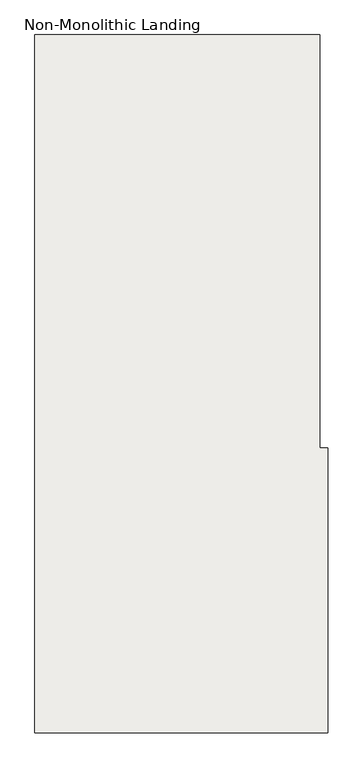
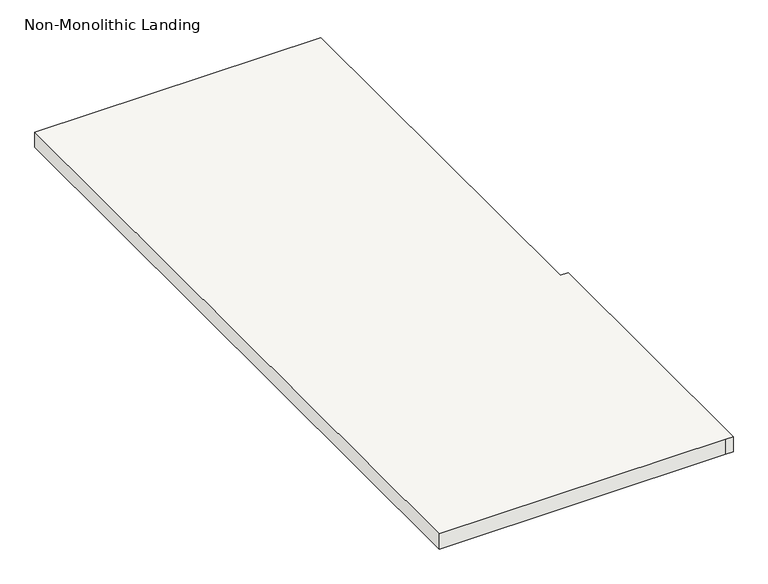
"""IFC4 building model written with IfcOpenShell, lengths in millimetres: slab geometry, Non-Monolithic Landing."""

from ifc_helpers import new_model, si_unit, origin, place, context, project, spatial, faceted_brep, source, transform, mapped, element, save


def non_monolithic_landing_62f4187a(model_context):
    return source(origin(), model_context, "Body", "Brep", [
        faceted_brep([(29538.0316163, 9282.3980552, 1987.55), (29563.4316163, 9282.3980552, 2012.95), (29563.4316163, 8367.9980552, 2012.95), (29538.0316163, 8367.9980552, 1987.55), (28649.0316163, 9282.3980552, 2032.0), (28649.0316163, 7040.8480552, 2032.0), (29563.4316163, 7040.8480552, 2032.0), (29588.8316163, 7040.8480552, 2032.0), (29588.8316163, 7955.2480552, 2032.0), (29563.4316163, 7955.2480552, 2032.0), (29563.4316163, 9282.3980552, 2032.0), (29538.0316163, 8367.9980552, 1981.2), (29563.4316163, 8367.9980552, 1981.2), (29563.4316163, 7955.2480552, 1981.2), (29588.8316163, 7955.2480552, 1981.2), (29588.8316163, 7040.8480552, 1981.2), (29563.4316163, 7040.8480552, 1981.2), (28649.0316163, 7040.8480552, 1981.2), (28649.0316163, 9282.3980552, 1981.2), (29538.0316163, 9282.3980552, 1981.2)], [[[0, 1, 2, 3]], [[4, 5, 6, 7, 8, 9, 10]], [[11, 12, 13, 14, 15, 16, 17, 18, 19]], [[12, 11, 3, 2]], [[11, 19, 0, 3]], [[4, 10, 1, 0, 19, 18]], [[5, 4, 18, 17]], [[6, 5, 17, 16]], [[7, 6, 16, 15]], [[8, 7, 15, 14]], [[9, 8, 14, 13]], [[10, 9, 13, 12, 2, 1]]]),
    ])


if __name__ == "__main__":
    model = new_model("IFC4")
    model_context = context("Model", 3, world=origin())
    ifc_project = project(units=[si_unit("LENGTHUNIT", "METRE", prefix="MILLI")], contexts=[model_context])
    site = spatial("IfcSite", under=ifc_project)
    building = spatial("IfcBuilding", under=site)
    placement = place(None, origin())
    non_monolithic_landing_shape = non_monolithic_landing_62f4187a(model_context)
    element("IfcSlab", 1, ObjectType="Non-Monolithic Landing", at=placement, inside=building, context=model_context, shape_type="MappedRepresentation", body=[
        mapped(non_monolithic_landing_shape, transform((0.0, 0.0, 0.0), x_axis=(1.0, 0.0, 0.0), y_axis=(0.0, 1.0, 0.0), z_axis=(0.0, 0.0, 1.0))),
    ])
    save(model, "model.ifc")
